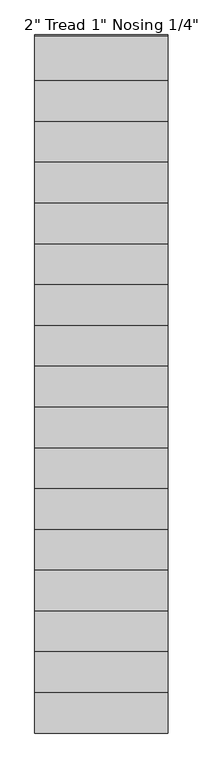
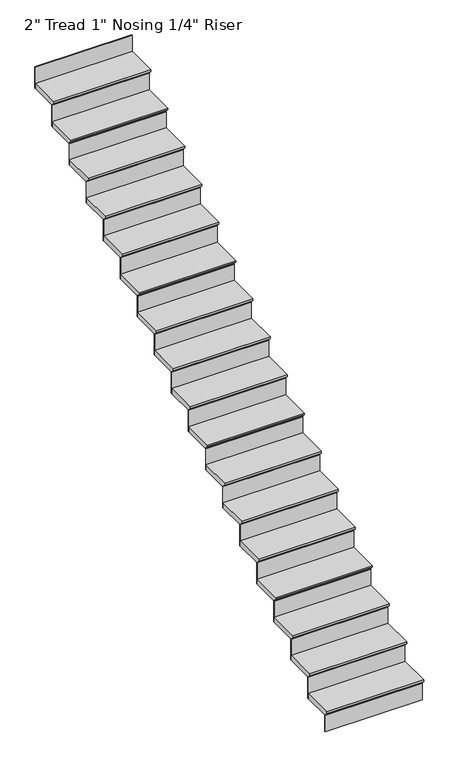
"""IFC4 building model written with IfcOpenShell, lengths in millimetres: stair flight geometry."""

from ifc_helpers import new_model, si_unit, frame, origin, origin_with_axes, place, context, project, spatial, polyline, outline, extrude, source, transform, mapped, element, save


def stair_flight_3767e4ab(model_context):
    return source(origin(), model_context, "Body", "SweptSolid", [
        extrude(outline(polyline([(3730.2992417, 211.6666667), (4035.0992417, 211.6666667), (4035.0992417, 160.8666667), (3755.6992417, 160.8666667), (3755.6992417, 167.2166667), (3730.2992417, 192.6166667), (3730.2992417, 211.6666667)])), frame((-6743.6917413, 0.0, 0.0), z_axis=(1.0, 0.0, 0.0), x_axis=(0.0, 1.0, 0.0)), (0.0, 0.0, 1.0), 914.4),
        extrude(outline(polyline([(-5829.2917413, 3762.0492417), (-5829.2917413, 3755.6992417), (-6743.6917413, 3755.6992417), (-6743.6917413, 3762.0492417), (-5829.2917413, 3762.0492417)])), origin_with_axes(), (0.0, 0.0, 1.0), 160.8666667),
        extrude(outline(polyline([(-5829.2917413, 4041.4492417), (-5829.2917413, 4035.0992417), (-6743.6917413, 4035.0992417), (-6743.6917413, 4041.4492417), (-5829.2917413, 4041.4492417)])), frame((0.0, 0.0, 160.8666667), z_axis=(0.0, 0.0, 1.0), x_axis=(1.0, 0.0, 0.0)), (0.0, 0.0, 1.0), 211.6666667),
        extrude(outline(polyline([(4009.6992417, 423.3333333), (4314.4992417, 423.3333333), (4314.4992417, 372.5333333), (4035.0992417, 372.5333333), (4035.0992417, 378.8833333), (4009.6992417, 404.2833333), (4009.6992417, 423.3333333)])), frame((-6743.6917413, 0.0, 0.0), z_axis=(1.0, 0.0, 0.0), x_axis=(0.0, 1.0, 0.0)), (0.0, 0.0, 1.0), 914.4),
        extrude(outline(polyline([(-5829.2917413, 4320.8492417), (-5829.2917413, 4314.4992417), (-6743.6917413, 4314.4992417), (-6743.6917413, 4320.8492417), (-5829.2917413, 4320.8492417)])), frame((0.0, 0.0, 372.5333333), z_axis=(0.0, 0.0, 1.0), x_axis=(1.0, 0.0, 0.0)), (0.0, 0.0, 1.0), 211.6666667),
        extrude(outline(polyline([(4289.0992417, 635.0), (4593.8992417, 635.0), (4593.8992417, 584.2), (4314.4992417, 584.2), (4314.4992417, 590.55), (4289.0992417, 615.95), (4289.0992417, 635.0)])), frame((-6743.6917413, 0.0, 0.0), z_axis=(1.0, 0.0, 0.0), x_axis=(0.0, 1.0, 0.0)), (0.0, 0.0, 1.0), 914.4),
        extrude(outline(polyline([(-5829.2917413, 4600.2492417), (-5829.2917413, 4593.8992417), (-6743.6917413, 4593.8992417), (-6743.6917413, 4600.2492417), (-5829.2917413, 4600.2492417)])), frame((0.0, 0.0, 584.2), z_axis=(0.0, 0.0, 1.0), x_axis=(1.0, 0.0, 0.0)), (0.0, 0.0, 1.0), 211.6666667),
        extrude(outline(polyline([(4568.4992417, 846.6666667), (4873.2992417, 846.6666667), (4873.2992417, 795.8666667), (4593.8992417, 795.8666667), (4593.8992417, 802.2166667), (4568.4992417, 827.6166667), (4568.4992417, 846.6666667)])), frame((-6743.6917413, 0.0, 0.0), z_axis=(1.0, 0.0, 0.0), x_axis=(0.0, 1.0, 0.0)), (0.0, 0.0, 1.0), 914.4),
        extrude(outline(polyline([(-5829.2917413, 4879.6492417), (-5829.2917413, 4873.2992417), (-6743.6917413, 4873.2992417), (-6743.6917413, 4879.6492417), (-5829.2917413, 4879.6492417)])), frame((0.0, 0.0, 795.8666667), z_axis=(0.0, 0.0, 1.0), x_axis=(1.0, 0.0, 0.0)), (0.0, 0.0, 1.0), 211.6666667),
        extrude(outline(polyline([(4847.8992417, 1058.3333333), (5152.6992417, 1058.3333333), (5152.6992417, 1007.5333333), (4873.2992417, 1007.5333333), (4873.2992417, 1013.8833333), (4847.8992417, 1039.2833333), (4847.8992417, 1058.3333333)])), frame((-6743.6917413, 0.0, 0.0), z_axis=(1.0, 0.0, 0.0), x_axis=(0.0, 1.0, 0.0)), (0.0, 0.0, 1.0), 914.4),
        extrude(outline(polyline([(-5829.2917413, 5159.0492417), (-5829.2917413, 5152.6992417), (-6743.6917413, 5152.6992417), (-6743.6917413, 5159.0492417), (-5829.2917413, 5159.0492417)])), frame((0.0, 0.0, 1007.5333333), z_axis=(0.0, 0.0, 1.0), x_axis=(1.0, 0.0, 0.0)), (0.0, 0.0, 1.0), 211.6666667),
        extrude(outline(polyline([(5127.2992417, 1270.0), (5432.0992417, 1270.0), (5432.0992417, 1219.2), (5152.6992417, 1219.2), (5152.6992417, 1225.55), (5127.2992417, 1250.95), (5127.2992417, 1270.0)])), frame((-6743.6917413, 0.0, 0.0), z_axis=(1.0, 0.0, 0.0), x_axis=(0.0, 1.0, 0.0)), (0.0, 0.0, 1.0), 914.4),
        extrude(outline(polyline([(-5829.2917413, 5438.4492417), (-5829.2917413, 5432.0992417), (-6743.6917413, 5432.0992417), (-6743.6917413, 5438.4492417), (-5829.2917413, 5438.4492417)])), frame((0.0, 0.0, 1219.2), z_axis=(0.0, 0.0, 1.0), x_axis=(1.0, 0.0, 0.0)), (0.0, 0.0, 1.0), 211.6666667),
        extrude(outline(polyline([(5406.6992417, 1481.6666667), (5711.4992417, 1481.6666667), (5711.4992417, 1430.8666667), (5432.0992417, 1430.8666667), (5432.0992417, 1437.2166667), (5406.6992417, 1462.6166667), (5406.6992417, 1481.6666667)])), frame((-6743.6917413, 0.0, 0.0), z_axis=(1.0, 0.0, 0.0), x_axis=(0.0, 1.0, 0.0)), (0.0, 0.0, 1.0), 914.4),
        extrude(outline(polyline([(-5829.2917413, 5717.8492417), (-5829.2917413, 5711.4992417), (-6743.6917413, 5711.4992417), (-6743.6917413, 5717.8492417), (-5829.2917413, 5717.8492417)])), frame((0.0, 0.0, 1430.8666667), z_axis=(0.0, 0.0, 1.0), x_axis=(1.0, 0.0, 0.0)), (0.0, 0.0, 1.0), 211.6666667),
        extrude(outline(polyline([(5686.0992417, 1693.3333333), (5990.8992417, 1693.3333333), (5990.8992417, 1642.5333333), (5711.4992417, 1642.5333333), (5711.4992417, 1648.8833333), (5686.0992417, 1674.2833333), (5686.0992417, 1693.3333333)])), frame((-6743.6917413, 0.0, 0.0), z_axis=(1.0, 0.0, 0.0), x_axis=(0.0, 1.0, 0.0)), (0.0, 0.0, 1.0), 914.4),
        extrude(outline(polyline([(-5829.2917413, 5997.2492417), (-5829.2917413, 5990.8992417), (-6743.6917413, 5990.8992417), (-6743.6917413, 5997.2492417), (-5829.2917413, 5997.2492417)])), frame((0.0, 0.0, 1642.5333333), z_axis=(0.0, 0.0, 1.0), x_axis=(1.0, 0.0, 0.0)), (0.0, 0.0, 1.0), 211.6666667),
        extrude(outline(polyline([(5965.4992417, 1905.0), (6270.2992417, 1905.0), (6270.2992417, 1854.2), (5990.8992417, 1854.2), (5990.8992417, 1860.55), (5965.4992417, 1885.95), (5965.4992417, 1905.0)])), frame((-6743.6917413, 0.0, 0.0), z_axis=(1.0, 0.0, 0.0), x_axis=(0.0, 1.0, 0.0)), (0.0, 0.0, 1.0), 914.4),
        extrude(outline(polyline([(-5829.2917413, 6276.6492417), (-5829.2917413, 6270.2992417), (-6743.6917413, 6270.2992417), (-6743.6917413, 6276.6492417), (-5829.2917413, 6276.6492417)])), frame((0.0, 0.0, 1854.2), z_axis=(0.0, 0.0, 1.0), x_axis=(1.0, 0.0, 0.0)), (0.0, 0.0, 1.0), 211.6666667),
        extrude(outline(polyline([(6244.8992417, 2116.6666667), (6549.6992417, 2116.6666667), (6549.6992417, 2065.8666667), (6270.2992417, 2065.8666667), (6270.2992417, 2072.2166667), (6244.8992417, 2097.6166667), (6244.8992417, 2116.6666667)])), frame((-6743.6917413, 0.0, 0.0), z_axis=(1.0, 0.0, 0.0), x_axis=(0.0, 1.0, 0.0)), (0.0, 0.0, 1.0), 914.4),
        extrude(outline(polyline([(-5829.2917413, 6556.0492417), (-5829.2917413, 6549.6992417), (-6743.6917413, 6549.6992417), (-6743.6917413, 6556.0492417), (-5829.2917413, 6556.0492417)])), frame((0.0, 0.0, 2065.8666667), z_axis=(0.0, 0.0, 1.0), x_axis=(1.0, 0.0, 0.0)), (0.0, 0.0, 1.0), 211.6666667),
        extrude(outline(polyline([(6524.2992417, 2328.3333333), (6829.0992417, 2328.3333333), (6829.0992417, 2277.5333333), (6549.6992417, 2277.5333333), (6549.6992417, 2283.8833333), (6524.2992417, 2309.2833333), (6524.2992417, 2328.3333333)])), frame((-6743.6917413, 0.0, 0.0), z_axis=(1.0, 0.0, 0.0), x_axis=(0.0, 1.0, 0.0)), (0.0, 0.0, 1.0), 914.4),
        extrude(outline(polyline([(-5829.2917413, 6835.4492417), (-5829.2917413, 6829.0992417), (-6743.6917413, 6829.0992417), (-6743.6917413, 6835.4492417), (-5829.2917413, 6835.4492417)])), frame((0.0, 0.0, 2277.5333333), z_axis=(0.0, 0.0, 1.0), x_axis=(1.0, 0.0, 0.0)), (0.0, 0.0, 1.0), 211.6666667),
        extrude(outline(polyline([(6803.6992417, 2540.0), (7108.4992417, 2540.0), (7108.4992417, 2489.2), (6829.0992417, 2489.2), (6829.0992417, 2495.55), (6803.6992417, 2520.95), (6803.6992417, 2540.0)])), frame((-6743.6917413, 0.0, 0.0), z_axis=(1.0, 0.0, 0.0), x_axis=(0.0, 1.0, 0.0)), (0.0, 0.0, 1.0), 914.4),
        extrude(outline(polyline([(-5829.2917413, 7114.8492417), (-5829.2917413, 7108.4992417), (-6743.6917413, 7108.4992417), (-6743.6917413, 7114.8492417), (-5829.2917413, 7114.8492417)])), frame((0.0, 0.0, 2489.2), z_axis=(0.0, 0.0, 1.0), x_axis=(1.0, 0.0, 0.0)), (0.0, 0.0, 1.0), 211.6666667),
        extrude(outline(polyline([(7083.0992417, 2751.6666667), (7387.8992417, 2751.6666667), (7387.8992417, 2700.8666667), (7108.4992417, 2700.8666667), (7108.4992417, 2707.2166667), (7083.0992417, 2732.6166667), (7083.0992417, 2751.6666667)])), frame((-6743.6917413, 0.0, 0.0), z_axis=(1.0, 0.0, 0.0), x_axis=(0.0, 1.0, 0.0)), (0.0, 0.0, 1.0), 914.4),
        extrude(outline(polyline([(-5829.2917413, 7394.2492417), (-5829.2917413, 7387.8992417), (-6743.6917413, 7387.8992417), (-6743.6917413, 7394.2492417), (-5829.2917413, 7394.2492417)])), frame((0.0, 0.0, 2700.8666667), z_axis=(0.0, 0.0, 1.0), x_axis=(1.0, 0.0, 0.0)), (0.0, 0.0, 1.0), 211.6666667),
        extrude(outline(polyline([(7362.4992417, 2963.3333333), (7667.2992417, 2963.3333333), (7667.2992417, 2912.5333333), (7387.8992417, 2912.5333333), (7387.8992417, 2918.8833333), (7362.4992417, 2944.2833333), (7362.4992417, 2963.3333333)])), frame((-6743.6917413, 0.0, 0.0), z_axis=(1.0, 0.0, 0.0), x_axis=(0.0, 1.0, 0.0)), (0.0, 0.0, 1.0), 914.4),
        extrude(outline(polyline([(-5829.2917413, 7673.6492417), (-5829.2917413, 7667.2992417), (-6743.6917413, 7667.2992417), (-6743.6917413, 7673.6492417), (-5829.2917413, 7673.6492417)])), frame((0.0, 0.0, 2912.5333333), z_axis=(0.0, 0.0, 1.0), x_axis=(1.0, 0.0, 0.0)), (0.0, 0.0, 1.0), 211.6666667),
        extrude(outline(polyline([(7641.8992417, 3175.0), (7946.6992417, 3175.0), (7946.6992417, 3124.2), (7667.2992417, 3124.2), (7667.2992417, 3130.55), (7641.8992417, 3155.95), (7641.8992417, 3175.0)])), frame((-6743.6917413, 0.0, 0.0), z_axis=(1.0, 0.0, 0.0), x_axis=(0.0, 1.0, 0.0)), (0.0, 0.0, 1.0), 914.4),
        extrude(outline(polyline([(-5829.2917413, 7953.0492417), (-5829.2917413, 7946.6992417), (-6743.6917413, 7946.6992417), (-6743.6917413, 7953.0492417), (-5829.2917413, 7953.0492417)])), frame((0.0, 0.0, 3124.2), z_axis=(0.0, 0.0, 1.0), x_axis=(1.0, 0.0, 0.0)), (0.0, 0.0, 1.0), 211.6666667),
        extrude(outline(polyline([(7921.2992417, 3386.6666667), (8226.0992417, 3386.6666667), (8226.0992417, 3335.8666667), (7946.6992417, 3335.8666667), (7946.6992417, 3342.2166667), (7921.2992417, 3367.6166667), (7921.2992417, 3386.6666667)])), frame((-6743.6917413, 0.0, 0.0), z_axis=(1.0, 0.0, 0.0), x_axis=(0.0, 1.0, 0.0)), (0.0, 0.0, 1.0), 914.4),
        extrude(outline(polyline([(-5829.2917413, 8232.4492417), (-5829.2917413, 8226.0992417), (-6743.6917413, 8226.0992417), (-6743.6917413, 8232.4492417), (-5829.2917413, 8232.4492417)])), frame((0.0, 0.0, 3335.8666667), z_axis=(0.0, 0.0, 1.0), x_axis=(1.0, 0.0, 0.0)), (0.0, 0.0, 1.0), 211.6666667),
        extrude(outline(polyline([(-5829.2917413, 8511.8492417), (-5829.2917413, 8505.4992417), (-6743.6917413, 8505.4992417), (-6743.6917413, 8511.8492417), (-5829.2917413, 8511.8492417)])), frame((0.0, 0.0, 3547.5333333), z_axis=(0.0, 0.0, 1.0), x_axis=(1.0, 0.0, 0.0)), (0.0, 0.0, 1.0), 211.6666667),
        extrude(outline(polyline([(8200.6992417, 3598.3333333), (8505.4992417, 3598.3333333), (8505.4992417, 3547.5333333), (8226.0992417, 3547.5333333), (8226.0992417, 3553.8833333), (8200.6992417, 3579.2833333), (8200.6992417, 3598.3333333)])), frame((-6743.6917413, 0.0, 0.0), z_axis=(1.0, 0.0, 0.0), x_axis=(0.0, 1.0, 0.0)), (0.0, 0.0, 1.0), 914.4),
    ])


if __name__ == "__main__":
    model = new_model("IFC4")
    model_context = context("Model", 3, world=origin())
    ifc_project = project(units=[si_unit("LENGTHUNIT", "METRE", prefix="MILLI")], contexts=[model_context])
    site = spatial("IfcSite", under=ifc_project)
    building = spatial("IfcBuilding", under=site)
    placement = place(None, origin())
    stair_flight_shape = stair_flight_3767e4ab(model_context)
    element("IfcStairFlight", 1, ObjectType="2\" Tread 1\" Nosing 1/4\" Riser", at=placement, inside=building, context=model_context, shape_type="MappedRepresentation", body=[
        mapped(stair_flight_shape, transform((0.0, 0.0, 0.0), x_axis=(1.0, 0.0, 0.0), y_axis=(0.0, 1.0, 0.0), z_axis=(0.0, 0.0, 1.0))),
    ])
    save(model, "model.ifc")
